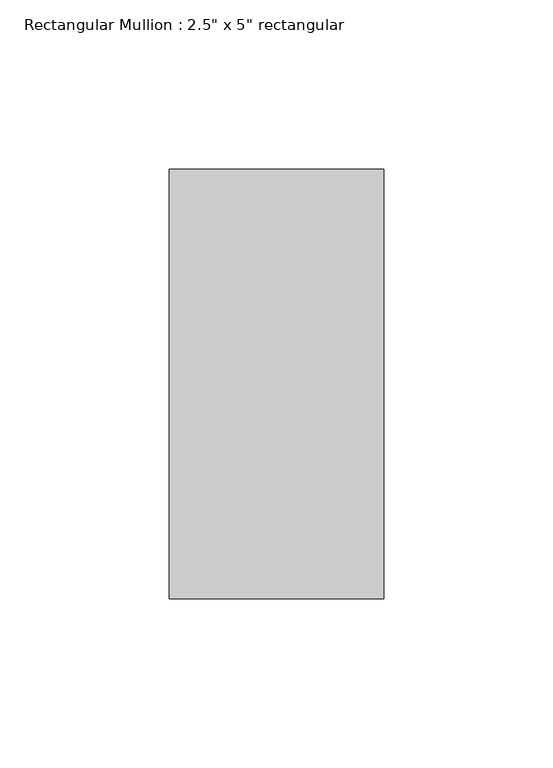
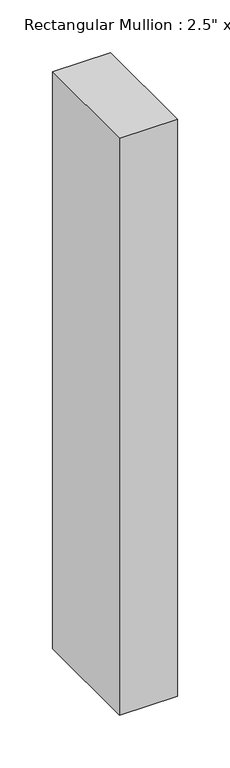
"""IFC4 building model written with IfcOpenShell, lengths in millimetres: member geometry."""

from ifc_helpers import new_model, si_unit, frame, origin, place, context, project, spatial, polyline, outline, extrude, source, transform, mapped, element, save


def member_9b03179d(model_context):
    return source(origin(), model_context, "Body", "SweptSolid", [
        extrude(outline(polyline([(0.0, 63.5), (0.0, -63.5), (-63.5, -63.5), (-63.5, 63.5), (0.0, 63.5)])), frame((0.0, 0.0, -667.8697067), z_axis=(0.0, 0.0, 1.0), x_axis=(1.0, 0.0, 0.0)), (0.0, 0.0, 1.0), 667.8697067),
    ])


if __name__ == "__main__":
    model = new_model("IFC4")
    model_context = context("Model", 3, world=origin())
    ifc_project = project(units=[si_unit("LENGTHUNIT", "METRE", prefix="MILLI")], contexts=[model_context])
    site = spatial("IfcSite", under=ifc_project)
    building = spatial("IfcBuilding", under=site)
    placement = place(None, origin())
    member_shape = member_9b03179d(model_context)
    element("IfcMember", 1, ObjectType="Rectangular Mullion : 2.5\" x 5\" rectangular", at=placement, inside=building, context=model_context, shape_type="MappedRepresentation", body=[
        mapped(member_shape, transform((0.0, 0.0, 0.0), x_axis=(1.0, 0.0, 0.0), y_axis=(0.0, 1.0, 0.0), z_axis=(0.0, 0.0, 1.0))),
    ])
    save(model, "model.ifc")

# Revit data of these elements
# Type "Rectangular Mullion : 2.5\" x 5\" rectangular"
#   built-in parameter 1007304 = 0.416667 (stored number, unit not read)
#   built-in parameter 1007301 = 0.104167 (stored number, unit not read)
#   built-in parameter 1007300 = 0.104167 (stored number, unit not read)
# Element 1 (IfcMember, "Rectangular Mullion : 2.5\" x 5\" rectangular")
#   Materials on its faces: "Aluminum"
# Materials
#   "Aluminum": class "Metal", colour RGB 247 247 247, transparency 0, Description = "Aluminum 6061", Cost = 0
